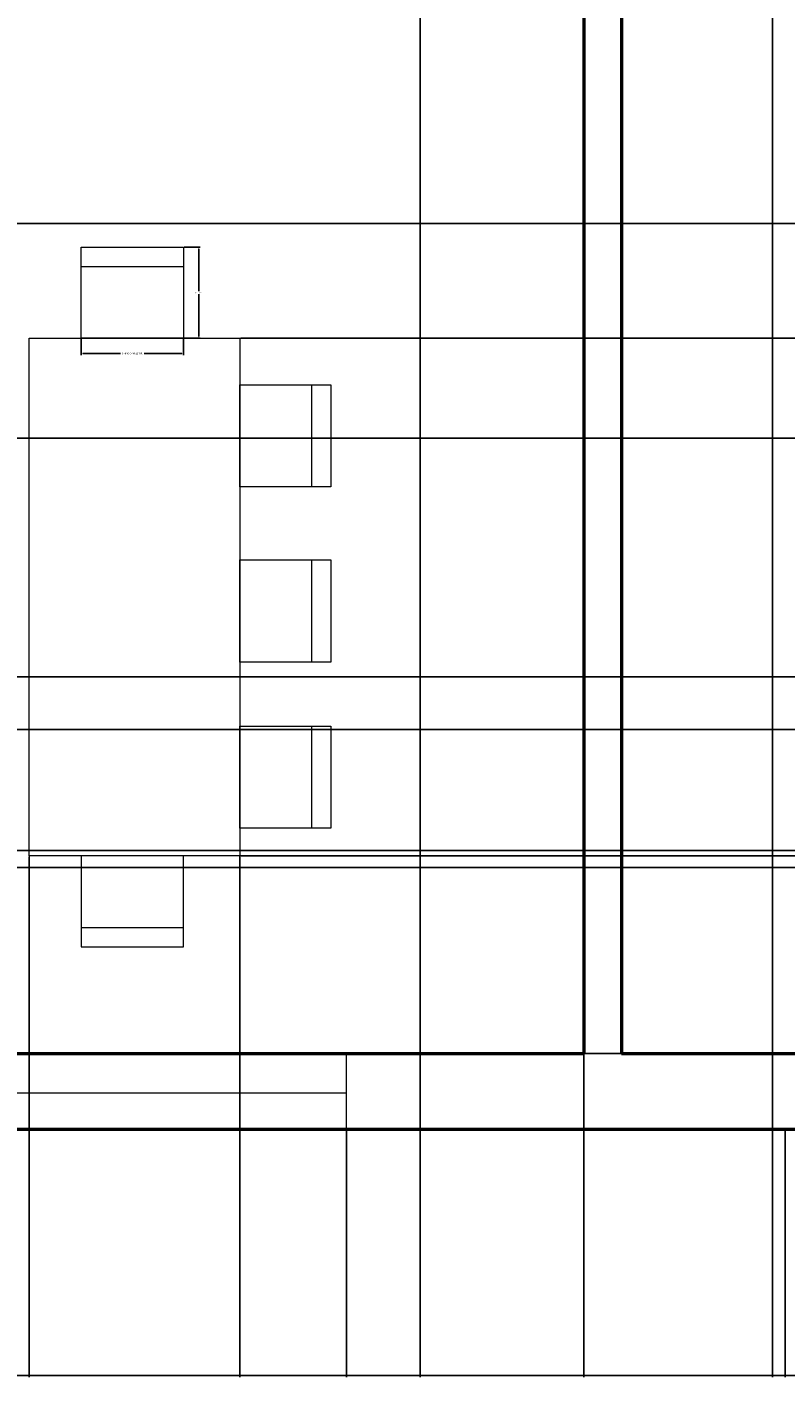
# Model space of a CAD drawing. Units: inches. Extents: x 19425 to 19848, y 45806 to 46417.
# Tile 2 of 5: x 19600 to 19690, y 45806 to 45967. Entities that reach past the tile are written whole.
import ezdxf

# ---------------------------------------------------------------- set-up
doc = ezdxf.new("R2010")
doc.units = ezdxf.units.IN
for name, color, linetype, lineweight in [('A-ANNO-DIMS', 2, 'Continuous', 18), ('furniture', 2, 'Continuous', 18), ('wall', 6, 'Continuous', 50), ('window', 9, 'Continuous', 20)]:
    doc.layers.add(name, color=color, linetype=linetype, lineweight=lineweight)
doc.styles.get("Standard").update_dxf_attribs({"font": 'arial.ttf'})
doc.dimstyles.get("Standard").update_dxf_attribs({"dimtxt": 0.18, "dimasz": 0.18, "dimexe": 0.18, "dimexo": 0.0625, "dimgap": 0.09, "dimtad": 0, "dimtih": 1, "dimtoh": 1, "dimdec": 4, "dimzin": 0, "dimdsep": 46, "dimtxsty": 'Standard', "dimcen": 0.09, "dimadec": 0, "dimazin": 0, "dimtfac": 1, "dimtdec": 4, "dimtofl": 0, "dimtmove": 0, "dimatfit": 3, "dimfxl": 1, "dimtolj": 1, "dimtzin": 0, "dimarcsym": 0})

# ---------------------------------------------------------------- blocks, each defined once
blk = doc.blocks.new('WIN-48-OFFSET-9')
for p, q in [((0, 0), (0, 9)), ((48, 0), (48, 9)), ((48, 4.28), (0, 4.28))]:
    blk.add_line(p, q)
blk = doc.blocks.new('CHAIR-DINING')
blk.add_line((0, 8.53), (12.17, 8.53))
blk.add_lwpolyline([(0, 10.82), (12.17, 10.82), (12.17, 0), (0, 0)], close=True)
blk = doc.blocks.new('*D14')
at = {"layer": 'A-ANNO-DIMS', "color": 0, "lineweight": -2, "transparency": 16777216}
for p, q in [((19606.41, 45929.89), (19606.41, 45927.94)), ((19618.58, 45929.89), (19618.58, 45927.94)), ((19606.59, 45928.12), (19611.07, 45928.12)), ((19618.4, 45928.12), (19613.92, 45928.12))]:
    blk.add_line(p, q, dxfattribs=at)
at = {"layer": 'A-ANNO-DIMS', "color": 0, "transparency": 16777216}
for points in [[(19606.59, 45928.15), (19606.59, 45928.09), (19606.41, 45928.12)], [(19618.4, 45928.15), (19618.4, 45928.09), (19618.58, 45928.12)]]:
    blk.add_solid(points, dxfattribs=at)
at = {"layer": 'Defpoints', "color": 0, "transparency": 16777216}
for p in [(19606.41, 45929.95), (19618.58, 45929.95), (19618.58, 45928.12)]:
    blk.add_point(p, dxfattribs=at)
at = {"layer": 'A-ANNO-DIMS', "color": 0, "transparency": 16777216, "insert": (19612.5, 45928.12), "char_height": 0.18, "attachment_point": 5}
blk.add_mtext('\\A1;DINING CHAIR 12 TYP.', dxfattribs=at)
blk = doc.blocks.new('*D15')
at = {"layer": 'A-ANNO-DIMS', "color": 0, "lineweight": -2, "transparency": 16777216}
for p, q in [((19618.65, 45940.77), (19620.59, 45940.77)), ((19620.41, 45940.59), (19620.41, 45935.54)), ((19620.41, 45930.13), (19620.41, 45935.18)), ((19618.65, 45929.95), (19620.59, 45929.95))]:
    blk.add_line(p, q, dxfattribs=at)
at = {"layer": 'A-ANNO-DIMS', "color": 0, "transparency": 16777216}
for points in [[(19620.38, 45940.59), (19620.44, 45940.59), (19620.41, 45940.77)], [(19620.38, 45930.13), (19620.44, 45930.13), (19620.41, 45929.95)]]:
    blk.add_solid(points, dxfattribs=at)
at = {"layer": 'Defpoints', "color": 0, "transparency": 16777216}
for p in [(19618.58, 45940.77), (19620.41, 45940.77), (19618.58, 45929.95)]:
    blk.add_point(p, dxfattribs=at)
at = {"layer": 'A-ANNO-DIMS', "color": 0, "transparency": 16777216, "insert": (19620.41, 45935.36), "char_height": 0.18, "attachment_point": 5}
blk.add_mtext('\\A1;11 TYP.', dxfattribs=at)
blk = doc.blocks.new('*D38')
at = {"layer": 'A-ANNO-DIMS', "color": 0, "lineweight": -2, "transparency": 16777216}
for p, q in [((19808.72, 45889.62), (19425.25, 45889.62)), ((19425.43, 45889.44), (19425.43, 45886.67)), ((19425.43, 45883.53), (19425.43, 45886.3)), ((19802.72, 45883.35), (19425.25, 45883.35))]:
    blk.add_line(p, q, dxfattribs=at)
at = {"layer": 'A-ANNO-DIMS', "color": 0, "transparency": 16777216}
for points in [[(19425.4, 45889.44), (19425.46, 45889.44), (19425.43, 45889.62)], [(19425.4, 45883.53), (19425.46, 45883.53), (19425.43, 45883.35)]]:
    blk.add_solid(points, dxfattribs=at)
at = {"layer": 'Defpoints', "color": 0, "transparency": 16777216}
for p in [(19425.43, 45889.62), (19808.78, 45889.62), (19802.78, 45883.35)]:
    blk.add_point(p, dxfattribs=at)
at = {"layer": 'A-ANNO-DIMS', "color": 0, "transparency": 16777216, "insert": (19425.43, 45886.49), "char_height": 0.18, "attachment_point": 5}
blk.add_mtext('\\A1;6.261', dxfattribs=at)
blk = doc.blocks.new('*D40')
at = {"layer": 'A-ANNO-DIMS', "color": 0, "lineweight": -2, "transparency": 16777216}
for p, q in [((19638, 45835.69), (19638, 45806.22)), ((19690.26, 45835.69), (19690.26, 45806.22)), ((19638.18, 45806.4), (19663.73, 45806.4)), ((19690.08, 45806.4), (19664.52, 45806.4))]:
    blk.add_line(p, q, dxfattribs=at)
at = {"layer": 'A-ANNO-DIMS', "color": 0, "transparency": 16777216}
for points in [[(19638.18, 45806.43), (19638.18, 45806.37), (19638, 45806.4)], [(19690.08, 45806.43), (19690.08, 45806.37), (19690.26, 45806.4)]]:
    blk.add_solid(points, dxfattribs=at)
at = {"layer": 'Defpoints', "color": 0, "transparency": 16777216}
for p in [(19638, 45835.75), (19690.26, 45835.75), (19690.26, 45806.4)]:
    blk.add_point(p, dxfattribs=at)
at = {"layer": 'A-ANNO-DIMS', "color": 0, "transparency": 16777216, "insert": (19664.13, 45806.4), "char_height": 0.18, "attachment_point": 5}
blk.add_mtext('\\A1;52.26', dxfattribs=at)
blk = doc.blocks.new('*D43')
at = {"layer": 'A-ANNO-DIMS', "color": 0, "lineweight": -2, "transparency": 16777216}
for p, q in [((19564.28, 45844.69), (19564.28, 45806.22)), ((19666.28, 45844.69), (19666.28, 45806.22)), ((19564.46, 45806.4), (19615, 45806.4)), ((19666.1, 45806.4), (19615.56, 45806.4))]:
    blk.add_line(p, q, dxfattribs=at)
at = {"layer": 'A-ANNO-DIMS', "color": 0, "transparency": 16777216}
for points in [[(19564.46, 45806.43), (19564.46, 45806.37), (19564.28, 45806.4)], [(19666.1, 45806.43), (19666.1, 45806.37), (19666.28, 45806.4)]]:
    blk.add_solid(points, dxfattribs=at)
at = {"layer": 'Defpoints', "color": 0, "transparency": 16777216}
for p in [(19564.28, 45844.75), (19666.28, 45844.75), (19666.28, 45806.4)]:
    blk.add_point(p, dxfattribs=at)
at = {"layer": 'A-ANNO-DIMS', "color": 0, "transparency": 16777216, "insert": (19615.28, 45806.4), "char_height": 0.18, "attachment_point": 5}
blk.add_mtext('\\A1;102', dxfattribs=at)
blk = doc.blocks.new('*D46')
at = {"layer": 'A-ANNO-DIMS', "color": 0, "lineweight": -2, "transparency": 16777216}
for p, q in [((19646.78, 46125.19), (19646.78, 45806.22)), ((19688.78, 46125.19), (19688.78, 45806.22)), ((19646.96, 45806.4), (19667.56, 45806.4)), ((19688.6, 45806.4), (19668, 45806.4))]:
    blk.add_line(p, q, dxfattribs=at)
at = {"layer": 'A-ANNO-DIMS', "color": 0, "transparency": 16777216}
for points in [[(19646.96, 45806.43), (19646.96, 45806.37), (19646.78, 45806.4)], [(19688.6, 45806.43), (19688.6, 45806.37), (19688.78, 45806.4)]]:
    blk.add_solid(points, dxfattribs=at)
at = {"layer": 'Defpoints', "color": 0, "transparency": 16777216}
for p in [(19646.78, 46125.25), (19688.78, 46125.25), (19688.78, 45806.4)]:
    blk.add_point(p, dxfattribs=at)
at = {"layer": 'A-ANNO-DIMS', "color": 0, "transparency": 16777216, "insert": (19667.78, 45806.4), "char_height": 0.18, "attachment_point": 5}
blk.add_mtext('\\A1;42', dxfattribs=at)
blk = doc.blocks.new('*D49')
at = {"layer": 'A-ANNO-DIMS', "color": 0, "lineweight": -2, "transparency": 16777216}
for p, q in [((19600.2, 45868.22), (19600.2, 45806.22)), ((19625.31, 45868.22), (19625.31, 45806.22)), ((19600.38, 45806.4), (19612.38, 45806.4)), ((19625.13, 45806.4), (19613.14, 45806.4))]:
    blk.add_line(p, q, dxfattribs=at)
at = {"layer": 'A-ANNO-DIMS', "color": 0, "transparency": 16777216}
for points in [[(19600.38, 45806.43), (19600.38, 45806.37), (19600.2, 45806.4)], [(19625.13, 45806.43), (19625.13, 45806.37), (19625.31, 45806.4)]]:
    blk.add_solid(points, dxfattribs=at)
at = {"layer": 'Defpoints', "color": 0, "transparency": 16777216}
for p in [(19600.2, 45868.28), (19625.31, 45868.28), (19625.31, 45806.4)]:
    blk.add_point(p, dxfattribs=at)
at = {"layer": 'A-ANNO-DIMS', "color": 0, "transparency": 16777216, "insert": (19612.76, 45806.4), "char_height": 0.18, "attachment_point": 5}
blk.add_mtext('\\A1;25.11', dxfattribs=at)
blk = doc.blocks.new('*D50')
at = {"layer": 'A-ANNO-DIMS', "color": 0, "lineweight": -2, "transparency": 16777216}
for p, q in [((19625.38, 45929.95), (19847.31, 45929.95)), ((19847.13, 45929.77), (19847.13, 45899.3)), ((19847.13, 45868.46), (19847.13, 45898.93)), ((19625.38, 45868.28), (19847.31, 45868.28))]:
    blk.add_line(p, q, dxfattribs=at)
at = {"layer": 'A-ANNO-DIMS', "color": 0, "transparency": 16777216}
for points in [[(19847.1, 45929.77), (19847.16, 45929.77), (19847.13, 45929.95)], [(19847.1, 45868.46), (19847.16, 45868.46), (19847.13, 45868.28)]]:
    blk.add_solid(points, dxfattribs=at)
at = {"layer": 'Defpoints', "color": 0, "transparency": 16777216}
for p in [(19625.31, 45929.95), (19847.13, 45929.95), (19625.31, 45868.28)]:
    blk.add_point(p, dxfattribs=at)
at = {"layer": 'A-ANNO-DIMS', "color": 0, "transparency": 16777216, "insert": (19847.13, 45899.11), "char_height": 0.18, "attachment_point": 5}
blk.add_mtext('\\A1;61.67', dxfattribs=at)
blk = doc.blocks.new('*D52')
at = {"layer": 'A-ANNO-DIMS', "color": 0, "lineweight": -2, "transparency": 16777216}
for p, q in [((19732.81, 46000.63), (19425.25, 46000.63)), ((19425.43, 46000.45), (19425.43, 45972.3)), ((19425.43, 45943.79), (19425.43, 45971.94)), ((19732.81, 45943.61), (19425.25, 45943.61))]:
    blk.add_line(p, q, dxfattribs=at)
at = {"layer": 'A-ANNO-DIMS', "color": 0, "transparency": 16777216}
for points in [[(19425.4, 46000.45), (19425.46, 46000.45), (19425.43, 46000.63)], [(19425.4, 45943.79), (19425.46, 45943.79), (19425.43, 45943.61)]]:
    blk.add_solid(points, dxfattribs=at)
at = {"layer": 'Defpoints', "color": 0, "transparency": 16777216}
for p in [(19425.43, 46000.63), (19732.87, 46000.63), (19732.87, 45943.61)]:
    blk.add_point(p, dxfattribs=at)
at = {"layer": 'A-ANNO-DIMS', "color": 0, "transparency": 16777216, "insert": (19425.43, 45972.12), "char_height": 0.18, "attachment_point": 5}
blk.add_mtext('\\A1;57.02', dxfattribs=at)
blk = doc.blocks.new('*D54')
at = {"layer": 'A-ANNO-DIMS', "color": 0, "lineweight": -2, "transparency": 16777216}
for p, q in [((19808.72, 46048.75), (19425.25, 46048.75)), ((19425.43, 46048.57), (19425.43, 45983.58)), ((19425.43, 45918.22), (19425.43, 45983.22)), ((19808.72, 45918.04), (19425.25, 45918.04))]:
    blk.add_line(p, q, dxfattribs=at)
at = {"layer": 'A-ANNO-DIMS', "color": 0, "transparency": 16777216}
for points in [[(19425.4, 46048.57), (19425.46, 46048.57), (19425.43, 46048.75)], [(19425.4, 45918.22), (19425.46, 45918.22), (19425.43, 45918.04)]]:
    blk.add_solid(points, dxfattribs=at)
at = {"layer": 'Defpoints', "color": 0, "transparency": 16777216}
for p in [(19425.43, 46048.75), (19808.78, 46048.75), (19808.78, 45918.04)]:
    blk.add_point(p, dxfattribs=at)
at = {"layer": 'A-ANNO-DIMS', "color": 0, "transparency": 16777216, "insert": (19425.43, 45983.4), "char_height": 0.18, "attachment_point": 5}
blk.add_mtext('\\A1;130.7', dxfattribs=at)
blk = doc.blocks.new('*D56')
at = {"layer": 'A-ANNO-DIMS', "color": 0, "lineweight": -2, "transparency": 16777216}
for p, q in [((19564.28, 45881.15), (19564.28, 45806.22)), ((19600.2, 45868.22), (19600.2, 45806.22)), ((19564.46, 45806.4), (19581.85, 45806.4)), ((19600.02, 45806.4), (19582.63, 45806.4))]:
    blk.add_line(p, q, dxfattribs=at)
at = {"layer": 'A-ANNO-DIMS', "color": 0, "transparency": 16777216}
for points in [[(19564.46, 45806.43), (19564.46, 45806.37), (19564.28, 45806.4)], [(19600.02, 45806.43), (19600.02, 45806.37), (19600.2, 45806.4)]]:
    blk.add_solid(points, dxfattribs=at)
at = {"layer": 'Defpoints', "color": 0, "transparency": 16777216}
for p in [(19564.28, 45881.22), (19600.2, 45868.28), (19600.2, 45806.4)]:
    blk.add_point(p, dxfattribs=at)
at = {"layer": 'A-ANNO-DIMS', "color": 0, "transparency": 16777216, "insert": (19582.24, 45806.4), "char_height": 0.18, "attachment_point": 5}
blk.add_mtext('\\A1;35.92', dxfattribs=at)
blk = doc.blocks.new('*D57')
at = {"layer": 'A-ANNO-DIMS', "color": 0, "lineweight": -2, "transparency": 16777216}
for p, q in [((19625.38, 45868.28), (19847.31, 45868.28)), ((19847.13, 45868.1), (19847.13, 45856.7)), ((19847.13, 45844.93), (19847.13, 45856.33)), ((19638.06, 45844.75), (19847.31, 45844.75))]:
    blk.add_line(p, q, dxfattribs=at)
at = {"layer": 'A-ANNO-DIMS', "color": 0, "transparency": 16777216}
for points in [[(19847.1, 45868.1), (19847.16, 45868.1), (19847.13, 45868.28)], [(19847.1, 45844.93), (19847.16, 45844.93), (19847.13, 45844.75)]]:
    blk.add_solid(points, dxfattribs=at)
at = {"layer": 'Defpoints', "color": 0, "transparency": 16777216}
for p in [(19625.31, 45868.28), (19638, 45844.75), (19847.13, 45844.75)]:
    blk.add_point(p, dxfattribs=at)
at = {"layer": 'A-ANNO-DIMS', "color": 0, "transparency": 16777216, "insert": (19847.13, 45856.52), "char_height": 0.18, "attachment_point": 5}
blk.add_mtext('\\A1;23.524', dxfattribs=at)
blk = doc.blocks.new('*D70')
at = {"layer": 'A-ANNO-DIMS', "color": 0, "lineweight": -2, "transparency": 16777216}
for p, q in [((19666.34, 45969.25), (19847.31, 45969.25)), ((19847.13, 45969.07), (19847.13, 45907.19)), ((19847.13, 45844.93), (19847.13, 45906.82)), ((19666.34, 45844.75), (19847.31, 45844.75))]:
    blk.add_line(p, q, dxfattribs=at)
at = {"layer": 'A-ANNO-DIMS', "color": 0, "transparency": 16777216}
for points in [[(19847.1, 45969.07), (19847.16, 45969.07), (19847.13, 45969.25)], [(19847.1, 45844.93), (19847.16, 45844.93), (19847.13, 45844.75)]]:
    blk.add_solid(points, dxfattribs=at)
at = {"layer": 'Defpoints', "color": 0, "transparency": 16777216}
for p in [(19666.28, 45969.25), (19847.13, 45969.25), (19666.28, 45844.75)]:
    blk.add_point(p, dxfattribs=at)
at = {"layer": 'A-ANNO-DIMS', "color": 0, "transparency": 16777216, "insert": (19847.13, 45907), "char_height": 0.18, "attachment_point": 5}
blk.add_mtext('\\A1;124.5', dxfattribs=at)
blk = doc.blocks.new('*D74')
at = {"layer": 'A-ANNO-DIMS', "color": 0, "lineweight": -2, "transparency": 16777216}
for p, q in [((19688.78, 46129.69), (19688.78, 45806.22)), ((19778.78, 46129.69), (19778.78, 45806.22)), ((19688.96, 45806.4), (19733.56, 45806.4)), ((19778.6, 45806.4), (19734, 45806.4))]:
    blk.add_line(p, q, dxfattribs=at)
at = {"layer": 'A-ANNO-DIMS', "color": 0, "transparency": 16777216}
for points in [[(19688.96, 45806.43), (19688.96, 45806.37), (19688.78, 45806.4)], [(19778.6, 45806.43), (19778.6, 45806.37), (19778.78, 45806.4)]]:
    blk.add_solid(points, dxfattribs=at)
at = {"layer": 'Defpoints', "color": 0, "transparency": 16777216}
for p in [(19688.78, 46129.75), (19778.78, 46129.75), (19778.78, 45806.4)]:
    blk.add_point(p, dxfattribs=at)
at = {"layer": 'A-ANNO-DIMS', "color": 0, "transparency": 16777216, "insert": (19733.78, 45806.4), "char_height": 0.18, "attachment_point": 5}
blk.add_mtext('\\A1;90', dxfattribs=at)
blk = doc.blocks.new('*D76')
at = {"layer": 'A-ANNO-DIMS', "color": 0, "lineweight": -2, "transparency": 16777216}
for p, q in [((19463.84, 45868.92), (19847.31, 45868.92)), ((19847.13, 45868.74), (19847.13, 45868.09)), ((19847.13, 45867.09), (19847.13, 45867.73)), ((19465.78, 45866.91), (19847.31, 45866.91))]:
    blk.add_line(p, q, dxfattribs=at)
at = {"layer": 'A-ANNO-DIMS', "color": 0, "transparency": 16777216}
for points in [[(19847.1, 45868.74), (19847.16, 45868.74), (19847.13, 45868.92)], [(19847.1, 45867.09), (19847.16, 45867.09), (19847.13, 45866.91)]]:
    blk.add_solid(points, dxfattribs=at)
at = {"layer": 'Defpoints', "color": 0, "transparency": 16777216}
for p in [(19463.78, 45868.92), (19465.72, 45866.91), (19847.13, 45866.91)]:
    blk.add_point(p, dxfattribs=at)
at = {"layer": 'A-ANNO-DIMS', "color": 0, "transparency": 16777216, "insert": (19847.13, 45867.91), "char_height": 0.18, "attachment_point": 5}
blk.add_mtext('\\A1;2.01', dxfattribs=at)

msp = doc.modelspace()

# ---------------------------------------------------------------- linework, layer by layer
at = {"layer": 'furniture'}
msp.add_lwpolyline([(19600.2018, 45929.95), (19625.3129, 45929.95), (19625.3129, 45868.2782), (19600.2018, 45868.2782)], close=True, dxfattribs=at)
at = {"layer": 'wall'}
for p, q in [((19666.2812, 45969.2547), (19666.2812, 45844.7547)), ((19670.7812, 45969.2547), (19670.7812, 45844.7547)), ((19564.2812, 45844.7547), (19666.2812, 45844.7547)), ((19670.7812, 45844.7547), (19760.7812, 45844.7547)), ((19454.7812, 45835.7547), (19760.7812, 45835.7547))]:
    msp.add_line(p, q, dxfattribs=at)

# ---------------------------------------------------------------- block references
at = {"layer": 'furniture'}
msp.add_blockref('CHAIR-DINING', (19606.4112, 45929.95), dxfattribs=at)
for p, rotation in [((19625.3129, 45924.3969), 270.0000000000002), ((19625.3129, 45903.5339), 269.9999999999703), ((19625.3129, 45883.7546), 269.9999999999703)]:
    msp.add_blockref('CHAIR-DINING', p, dxfattribs=dict(at, rotation=rotation))
at = {"layer": 'furniture', "extrusion": (0, 0, -1), "zscale": -1, "rotation": 180}
msp.add_blockref('CHAIR-DINING', (-19606.4112, 45868.2782), dxfattribs=at)
at = {"layer": 'window'}
msp.add_blockref('WIN-48-OFFSET-9', (19589.9971, 45835.7547), dxfattribs=at)

# ---------------------------------------------------------------- dimensions: what is measured, and where the dimension line sits
at = {"layer": 'A-ANNO-DIMS'}
for base, p1, p2, override, picture, middle in [((19778.7812, 45806.4047), (19688.7812, 46129.7547), (19778.7812, 46129.7547), {"dimdec": 0, "dimlfac": 1, "dimrnd": 0, "dimzin": 0, "dimdsep": 46, "dimlunit": 2}, '*D74', (19733.7812, 45806.4047)), ((19688.7812, 45806.4047), (19646.7812, 46125.2547), (19688.7812, 46125.2547), {"dimdec": 0, "dimlfac": 1, "dimrnd": 0, "dimzin": 0, "dimdsep": 46, "dimlunit": 2}, '*D46', (19667.7812, 45806.4047)), ((19600.2018, 45806.4047), (19564.2812, 45881.2164), (19600.2018, 45868.2782), {"dimdec": 2, "dimlfac": 1, "dimrnd": 0, "dimzin": 0, "dimdsep": 46, "dimlunit": 2}, '*D56', (19582.2415, 45806.4047)), ((19625.3129, 45806.4047), (19600.2018, 45868.2782), (19625.3129, 45868.2782), {"dimdec": 2, "dimlfac": 1, "dimrnd": 0, "dimzin": 0, "dimdsep": 46, "dimlunit": 2}, '*D49', (19612.7573, 45806.4047)), ((19666.2812, 45806.4047), (19564.2812, 45844.7547), (19666.2812, 45844.7547), {"dimdec": 0, "dimlfac": 1, "dimrnd": 0, "dimzin": 0, "dimdsep": 46, "dimlunit": 2}, '*D43', (19615.2812, 45806.4047)), ((19690.2556, 45806.4047), (19637.9971, 45835.7547), (19690.2556, 45835.7547), {"dimdec": 2, "dimlfac": 1, "dimrnd": 0, "dimzin": 0, "dimdsep": 46, "dimlunit": 2}, '*D40', (19664.1264, 45806.4047))]:
    dim = msp.add_linear_dim(base=base, p1=p1, p2=p2, dimstyle='Standard', override=override, dxfattribs=at)
    dim.commit()
    dim.dimension.update_dxf_attribs({"geometry": picture, "text_midpoint": middle})
for base, p1, p2, override, picture, middle in [((19425.4312, 46048.7547), (19808.7812, 45918.0438), (19808.7812, 46048.7547), {"dimdec": 1, "dimlfac": 1, "dimrnd": 0, "dimzin": 0, "dimdsep": 46, "dimlunit": 2}, '*D54', (19425.4312, 45983.3992)), ((19425.4312, 46000.631), (19732.8741, 45943.6092), (19732.8741, 46000.631), {"dimdec": 2, "dimlfac": 1, "dimrnd": 0, "dimzin": 0, "dimdsep": 46, "dimlunit": 2}, '*D52', (19425.4312, 45972.1201)), ((19847.1312, 45969.2547), (19666.2812, 45844.7547), (19666.2812, 45969.2547), {"dimdec": 1, "dimlfac": 1, "dimrnd": 0, "dimzin": 0, "dimdsep": 46, "dimlunit": 2}, '*D70', (19847.1312, 45907.0047)), ((19847.1312, 45929.95), (19625.3129, 45868.2782), (19625.3129, 45929.95), {"dimdec": 2, "dimlfac": 1, "dimrnd": 0, "dimzin": 0, "dimdsep": 46, "dimlunit": 2}, '*D50', (19847.1312, 45899.1141)), ((19425.4312, 45889.6159), (19802.7812, 45883.3547), (19808.7812, 45889.6159), {"dimdec": 3, "dimlfac": 1, "dimrnd": 0, "dimzin": 0, "dimdsep": 46, "dimlunit": 2}, '*D38', (19425.4312, 45886.4853)), ((19847.1312, 45866.9088), (19463.7812, 45868.9163), (19465.7192, 45866.9088), {"dimdec": 2, "dimlfac": 1, "dimrnd": 0, "dimzin": 0, "dimdsep": 46, "dimlunit": 2}, '*D76', (19847.1312, 45867.9126)), ((19847.13116, 45844.75465), (19625.31287, 45868.27825), (19637.99712, 45844.75465), {"dimdec": 3, "dimlfac": 1, "dimrnd": 0, "dimzin": 0, "dimdsep": 46, "dimlunit": 2}, '*D57', (19847.13116, 45856.51645))]:
    dim = msp.add_linear_dim(base=base, p1=p1, p2=p2, angle=90, dimstyle='Standard', override=override, dxfattribs=at)
    dim.commit()
    dim.dimension.update_dxf_attribs({"geometry": picture, "text_midpoint": middle})
dim = msp.add_linear_dim(base=(19620.4104, 45940.7688), p1=(19618.5844, 45929.95), p2=(19618.5844, 45940.7688), angle=90, text='<> TYP.', dimstyle='Standard', override={"dimdec": 0, "dimlfac": 1, "dimrnd": 0, "dimzin": 0, "dimdsep": 46, "dimlunit": 2}, dxfattribs=at)
dim.commit()
dim.dimension.update_dxf_attribs({"geometry": '*D15', "text_midpoint": (19620.4104, 45935.3594)})
dim = msp.add_linear_dim(base=(19618.5844, 45928.124), p1=(19606.4112, 45929.95), p2=(19618.5844, 45929.95), text='DINING CHAIR <> TYP.', dimstyle='Standard', override={"dimdec": 0, "dimlfac": 1, "dimrnd": 0, "dimzin": 0, "dimdsep": 46, "dimlunit": 2}, dxfattribs=at)
dim.commit()
dim.dimension.update_dxf_attribs({"geometry": '*D14', "text_midpoint": (19612.4978, 45928.124)})

doc.saveas('drawing.dxf')
